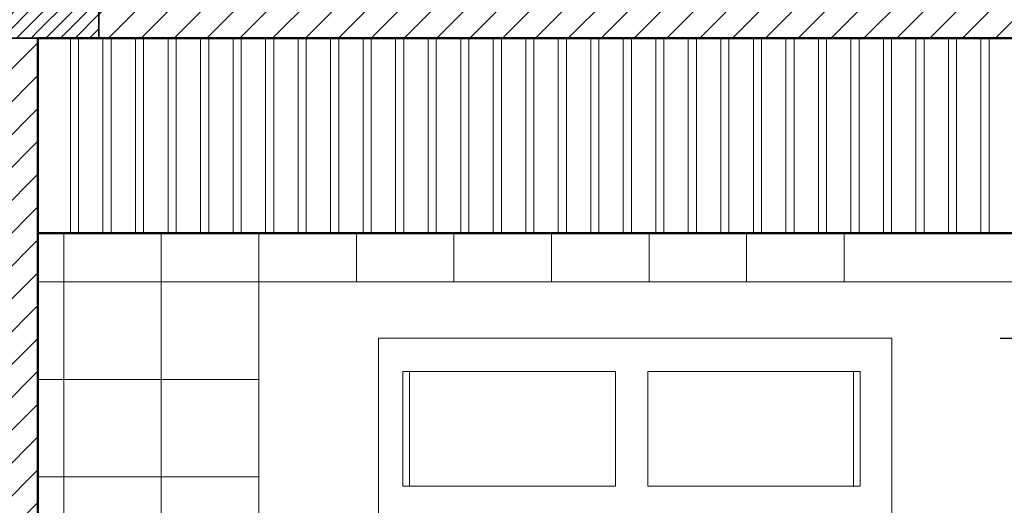
# Model space of a CAD drawing. Units: millimetres. Extents: x 225995 to 227247, y 225507 to 226008.
# Tile 21 of 23: x 227029 to 227150, y 225868 to 225928. Entities that reach past the tile are written whole.
import ezdxf

# ---------------------------------------------------------------- set-up
doc = ezdxf.new("R2010")
doc.units = ezdxf.units.MM
for name, color, linetype, lineweight in [('A-ANNO-DIMS', 2, 'Continuous', 18), ('A-COLS', 40, 'Continuous', 35), ('A-FLOR-PATT', 8, 'Continuous', 13), ('A-FURN', 9, 'Continuous', 18), ('A-WALL', 7, 'Continuous', 50), ('A-WALL-PATT', 8, 'Continuous', 13)]:
    doc.layers.add(name, color=color, linetype=linetype, lineweight=lineweight)
doc.styles.get("Standard").update_dxf_attribs({"font": 'arial.ttf'})
doc.dimstyles.new('ISO-25', dxfattribs={"dimtxt": 6, "dimasz": 2.5, "dimexe": 1.25, "dimexo": 0.625, "dimtad": 1, "dimdec": 0, "dimlunit": 3, "dimtxsty": 'Standard', "dimcen": 2.5, "dimadec": 0, "dimazin": 0, "dimtfac": 1, "dimtdec": 0, "dimtmove": 0, "dimatfit": 3, "dimfxl": 1, "dimarcsym": 0})
pattern_1 = [(45, (646.0463, 0.931), (-2.020557627, 2.020557627), [])]
pattern_2 = [(45, (646.0463, 234.931), (-0.898025612, 0.898025612), [])]

# ---------------------------------------------------------------- blocks, each defined once
blk = doc.blocks.new('A$C6D2A2628')
for p, q in [((0.291, 2.4297), (1.791, 2.4297)), ((0.291, 0.4297), (0.291, 2.4297)), ((1.791, 2.4297), (1.791, 0.4297)), ((0.3622, 2.3321), (0.9834, 2.3321)), ((0.3622, 1.9967), (0.3622, 2.3321)), ((0.3822, 1.9967), (0.3822, 2.3321)), ((0.9834, 2.3321), (0.9834, 1.9967)), ((1.0779, 2.3321), (1.6991, 2.3321)), ((1.0779, 1.9967), (1.0779, 2.3321)), ((1.6791, 2.3321), (1.6791, 1.9967)), ((1.6991, 2.3321), (1.6991, 1.9967)), ((0.9834, 1.9967), (0.3622, 1.9967)), ((1.6991, 1.9967), (1.0779, 1.9967))]:
    blk.add_line(p, q)
blk = doc.blocks.new('*D79')
at = {"layer": 'A-ANNO-DIMS', "color": 0, "lineweight": -2, "transparency": 16777216}
for p, q in [((227149.28, 225888.79), (227165.25, 225888.79)), ((227164, 225789.02), (227164, 225886.29)), ((227149.28, 225786.52), (227165.25, 225786.52))]:
    blk.add_line(p, q, dxfattribs=at)
at = {"layer": 'A-ANNO-DIMS', "color": 0, "transparency": 16777216}
for points in [[(227163.58, 225886.29), (227164.41, 225886.29), (227164, 225888.79)], [(227163.58, 225789.02), (227164.41, 225789.02), (227164, 225786.52)]]:
    blk.add_solid(points, dxfattribs=at)
at = {"layer": 'Defpoints', "color": 0, "transparency": 16777216}
for p in [(227148.66, 225888.79), (227164, 225888.79), (227148.66, 225786.52)]:
    blk.add_point(p, dxfattribs=at)
at = {"layer": 'A-ANNO-DIMS', "color": 0, "transparency": 16777216, "insert": (227160.27, 225837.65), "char_height": 6, "attachment_point": 5, "rotation": 90}
blk.add_mtext('BED 8\'-6 1/2" TYP.', dxfattribs=at)

msp = doc.modelspace()

# ---------------------------------------------------------------- hatches: boundary and pattern name
at = {"layer": 'A-WALL-PATT'}
h = msp.add_hatch(dxfattribs=at)
h.set_pattern_fill('ANSI31', color=256, scale=0.9)
h.set_pattern_definition(pattern_1)
h.paths.add_polyline_path([(227167.42, 225934.7), (227038.42, 225934.7), (227038.42, 225925.7), (227167.42, 225925.7)])
h = msp.add_hatch(dxfattribs=at)
h.set_pattern_fill('ANSI31', color=256, scale=0.4)
h.set_pattern_definition(pattern_2)
h.paths.add_polyline_path([(227030.92, 225930.2), (227026.42, 225930.2), (227026.42, 225925.7), (227030.92, 225925.7)])
h = msp.add_hatch(dxfattribs=at)
h.set_pattern_fill('ANSI31', color=256, scale=0.4)
h.set_pattern_definition(pattern_2)
h.paths.add_polyline_path([(227038.42, 225930.2), (227030.92, 225930.2), (227030.92, 225925.7), (227038.42, 225925.7)])
h = msp.add_hatch(dxfattribs=at)
h.set_pattern_fill('ANSI31', color=256, scale=0.9)
h.set_pattern_definition(pattern_1)
h.paths.add_polyline_path([(227030.92, 225925.7), (227026.42, 225925.7), (227026.42, 225818.84), (227030.92, 225818.84)])

# ---------------------------------------------------------------- linework, layer by layer
at = {"layer": 'A-COLS'}
msp.add_lwpolyline([(227026.42, 225925.7), (227026.42, 225934.7), (227038.42, 225934.7), (227038.42, 225925.7)], close=True, dxfattribs=at)
at = {"layer": 'A-FLOR-PATT'}
for p, q in [((227034.09, 225901.7), (227034.09, 225818.84)), ((227046.09, 225901.7), (227046.09, 225696.2)), ((227058.09, 225901.7), (227058.09, 225696.2)), ((227070.09, 225901.7), (227070.09, 225895.7)), ((227082.09, 225901.7), (227082.09, 225895.7)), ((227094.09, 225901.7), (227094.09, 225895.7)), ((227106.09, 225901.7), (227106.09, 225895.7)), ((227118.09, 225901.7), (227118.09, 225895.7)), ((227130.09, 225901.7), (227130.09, 225895.7)), ((227030.92, 225895.7), (227203.42, 225895.7)), ((227030.92, 225883.7), (227058.09, 225883.7)), ((227030.92, 225871.7), (227058.09, 225871.7))]:
    msp.add_line(p, q, dxfattribs=at)
at = {"layer": 'A-FURN'}
for p, q in [((227034.92, 225901.7), (227034.92, 225925.7)), ((227035.92, 225901.7), (227035.92, 225925.7)), ((227038.92, 225901.7), (227038.92, 225925.7)), ((227039.92, 225901.7), (227039.92, 225925.7)), ((227042.92, 225901.7), (227042.92, 225925.7)), ((227043.92, 225901.7), (227043.92, 225925.7)), ((227046.92, 225901.7), (227046.92, 225925.7)), ((227047.92, 225901.7), (227047.92, 225925.7)), ((227050.92, 225901.7), (227050.92, 225925.7)), ((227051.92, 225901.7), (227051.92, 225925.7)), ((227054.92, 225901.7), (227054.92, 225925.7)), ((227055.92, 225901.7), (227055.92, 225925.7)), ((227058.92, 225901.7), (227058.92, 225925.7)), ((227059.92, 225901.7), (227059.92, 225925.7)), ((227062.92, 225901.7), (227062.92, 225925.7)), ((227063.92, 225901.7), (227063.92, 225925.7)), ((227066.92, 225901.7), (227066.92, 225925.7)), ((227067.92, 225901.7), (227067.92, 225925.7)), ((227070.92, 225901.7), (227070.92, 225925.7)), ((227071.92, 225901.7), (227071.92, 225925.7)), ((227074.92, 225901.7), (227074.92, 225925.7)), ((227075.92, 225901.7), (227075.92, 225925.7)), ((227078.92, 225901.7), (227078.92, 225925.7)), ((227079.92, 225901.7), (227079.92, 225925.7)), ((227082.92, 225901.7), (227082.92, 225925.7)), ((227083.92, 225901.7), (227083.92, 225925.7)), ((227086.92, 225901.7), (227086.92, 225925.7)), ((227087.92, 225901.7), (227087.92, 225925.7)), ((227090.92, 225901.7), (227090.92, 225925.7)), ((227091.92, 225901.7), (227091.92, 225925.7)), ((227094.92, 225901.7), (227094.92, 225925.7)), ((227095.92, 225901.7), (227095.92, 225925.7)), ((227098.92, 225901.7), (227098.92, 225925.7)), ((227099.92, 225901.7), (227099.92, 225925.7)), ((227102.92, 225901.7), (227102.92, 225925.7)), ((227103.92, 225901.7), (227103.92, 225925.7)), ((227106.92, 225901.7), (227106.92, 225925.7)), ((227107.92, 225901.7), (227107.92, 225925.7)), ((227110.92, 225901.7), (227110.92, 225925.7)), ((227111.92, 225901.7), (227111.92, 225925.7)), ((227114.92, 225901.7), (227114.92, 225925.7)), ((227115.92, 225901.7), (227115.92, 225925.7)), ((227118.92, 225901.7), (227118.92, 225925.7)), ((227119.92, 225901.7), (227119.92, 225925.7)), ((227122.92, 225901.7), (227122.92, 225925.7)), ((227123.92, 225901.7), (227123.92, 225925.7)), ((227126.92, 225901.7), (227126.92, 225925.7)), ((227127.92, 225901.7), (227127.92, 225925.7)), ((227130.92, 225901.7), (227130.92, 225925.7)), ((227131.92, 225901.7), (227131.92, 225925.7)), ((227134.92, 225901.7), (227134.92, 225925.7)), ((227135.92, 225901.7), (227135.92, 225925.7)), ((227138.92, 225901.7), (227138.92, 225925.7)), ((227139.92, 225901.7), (227139.92, 225925.7)), ((227142.92, 225901.7), (227142.92, 225925.7)), ((227143.92, 225901.7), (227143.92, 225925.7)), ((227146.92, 225901.7), (227146.92, 225925.7)), ((227147.92, 225901.7), (227147.92, 225925.7))]:
    msp.add_line(p, q, dxfattribs=at)
at = {"layer": 'A-WALL'}
for p, q in [((227030.92, 225925.7), (227203.42, 225925.7)), ((227030.92, 225741.2), (227030.92, 225925.7)), ((227203.42, 225925.7), (227030.92, 225925.7)), ((227030.92, 225925.7), (227030.92, 225741.2)), ((227030.92, 225901.7), (227203.42, 225901.7))]:
    msp.add_line(p, q, dxfattribs=at)

# ---------------------------------------------------------------- block references
at = {"layer": 'A-FURN', "xscale": 42.09102840542158, "yscale": 42.09102840542158, "zscale": 42.09102840542158}
msp.add_blockref('A$C6D2A2628', (227060.55, 225786.52), dxfattribs=at)

# ---------------------------------------------------------------- dimensions: what is measured, and where the dimension line sits
at = {"layer": 'A-ANNO-DIMS'}
dim = msp.add_linear_dim(base=(227164, 225888.79), p1=(227148.66, 225786.52), p2=(227148.66, 225888.79), angle=90, text='BED <> TYP.', dimstyle='ISO-25', override={"dimdec": 1, "dimrnd": 0, "dimzin": 1, "dimlunit": 4, "dimfrac": 2}, dxfattribs=at)
dim.commit()
dim.dimension.update_dxf_attribs({"geometry": '*D79', "text_midpoint": (227160.27, 225837.65)})

doc.saveas('drawing.dxf')
